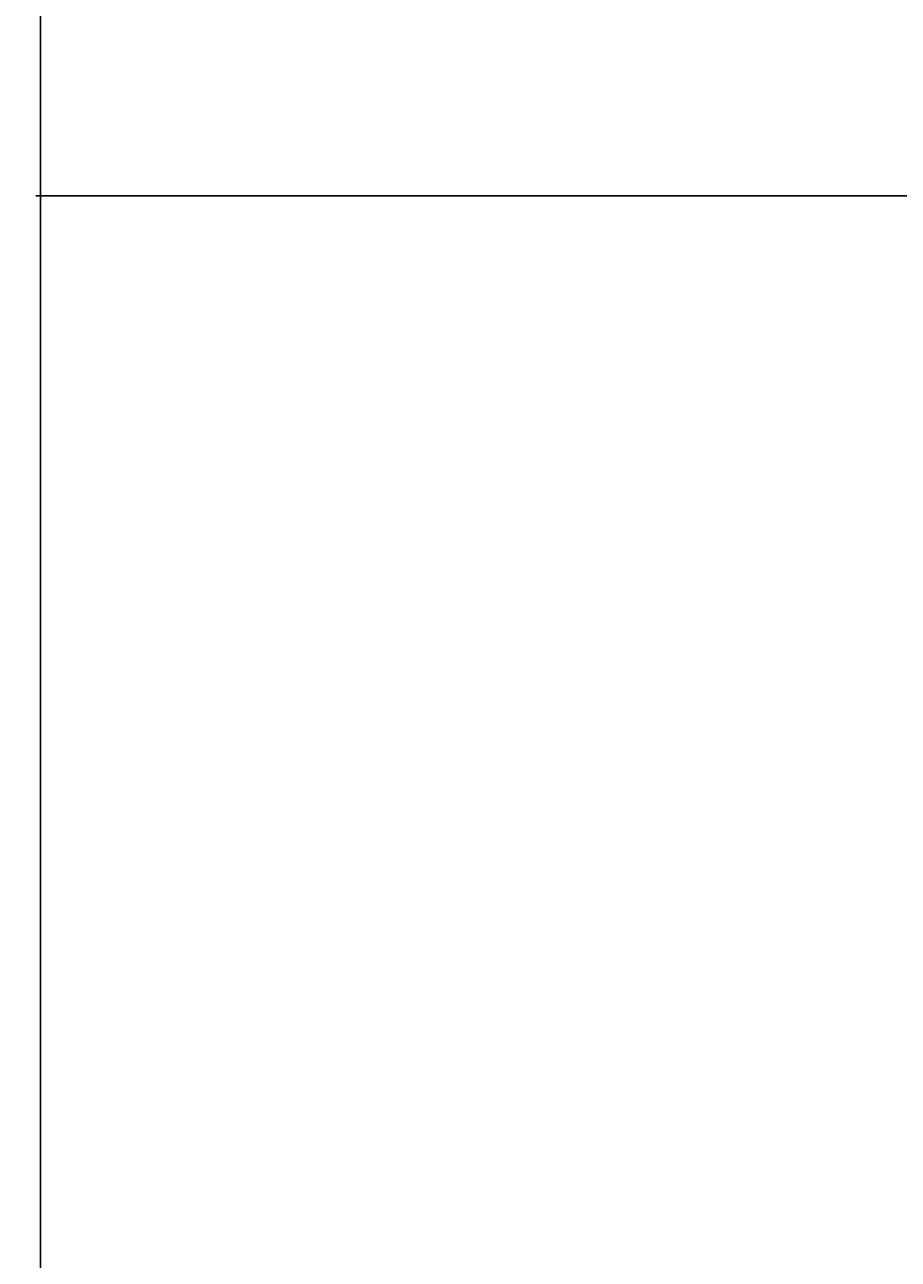
# Model space of a CAD drawing. Units: inches. Extents: x -301 to 715, y -607 to 364.
# Tile 96 of 141: x 161 to 194, y -124 to -77. Entities that reach past the tile are written whole.
import ezdxf

# ---------------------------------------------------------------- set-up
doc = ezdxf.new("R2010")
doc.units = ezdxf.units.IN
doc.header["$MEASUREMENT"] = 0
doc.layers.add('A-ANNO-DIMS', color=2, linetype='Continuous', lineweight=18)
doc.styles.get("Standard").update_dxf_attribs({"font": 'arial.ttf'})
doc.dimstyles.get("Standard").update_dxf_attribs({"dimtxt": 0.18, "dimasz": 0.18, "dimexe": 0.18, "dimexo": 0.0625, "dimgap": 0.09, "dimtad": 0, "dimtih": 1, "dimtoh": 1, "dimdec": 1, "dimzin": 0, "dimdsep": 46, "dimlunit": 4, "dimtxsty": 'Standard', "dimcen": 0.09, "dimclrd": 3, "dimclre": 4, "dimclrt": 6, "dimadec": 0, "dimazin": 0, "dimtfac": 1, "dimtdec": 1, "dimtofl": 0, "dimtmove": 0, "dimatfit": 3, "dimfxl": 1, "dimtfill": 2, "dimtfillclr": 51, "dimtolj": 1, "dimtzin": 0, "dimarcsym": 0})

# ---------------------------------------------------------------- blocks, each defined once
blk = doc.blocks.new('*D162')
at = {"layer": 'A-ANNO-DIMS', "color": 4, "lineweight": -2, "transparency": 16777216}
for p, q in [((222.328, 320.182), (161.439, 320.182)), ((222.328, -233.818), (161.439, -233.818))]:
    blk.add_line(p, q, dxfattribs=at)
at = {"layer": 'A-ANNO-DIMS', "color": 3, "lineweight": -2, "transparency": 16777216}
for p, q in [((161.619, 320.002), (161.619, 43.364)), ((161.619, -233.638), (161.619, 43))]:
    blk.add_line(p, q, dxfattribs=at)
at = {"layer": 'A-ANNO-DIMS', "color": 3, "transparency": 16777216}
for points in [[(161.589, 320.002), (161.649, 320.002), (161.619, 320.182)], [(161.589, -233.638), (161.649, -233.638), (161.619, -233.818)]]:
    blk.add_solid(points, dxfattribs=at)
at = {"layer": 'Defpoints', "color": 0, "transparency": 16777216}
for p in [(161.619, 320.182), (222.39, 320.182), (222.39, -233.818)]:
    blk.add_point(p, dxfattribs=at)
at = {"layer": 'A-ANNO-DIMS', "color": 6, "transparency": 16777216, "insert": (161.619, 43.182), "char_height": 0.18, "attachment_point": 5, "bg_fill": 1, "box_fill_scale": 1.25, "bg_fill_color": 51, "bg_fill_transparency": 0}
blk.add_mtext('\\A1;46\'-2"', dxfattribs=at)
blk = doc.blocks.new('*D167')
at = {"layer": 'A-ANNO-DIMS', "color": 4, "lineweight": -2, "transparency": 16777216}
for p, q in [((222.328, -83.318), (161.439, -83.318)), ((222.328, -233.818), (161.439, -233.818))]:
    blk.add_line(p, q, dxfattribs=at)
at = {"layer": 'A-ANNO-DIMS', "color": 3, "lineweight": -2, "transparency": 16777216}
for p, q in [((161.619, -83.498), (161.619, -158.385)), ((161.619, -233.638), (161.619, -158.751))]:
    blk.add_line(p, q, dxfattribs=at)
at = {"layer": 'A-ANNO-DIMS', "color": 3, "transparency": 16777216}
for points in [[(161.589, -83.498), (161.649, -83.498), (161.619, -83.318)], [(161.589, -233.638), (161.649, -233.638), (161.619, -233.818)]]:
    blk.add_solid(points, dxfattribs=at)
at = {"layer": 'Defpoints', "color": 0, "transparency": 16777216}
for p in [(161.619, -83.318), (222.39, -83.318), (222.39, -233.818)]:
    blk.add_point(p, dxfattribs=at)
at = {"layer": 'A-ANNO-DIMS', "color": 6, "transparency": 16777216, "insert": (161.619, -158.568), "char_height": 0.18, "attachment_point": 5, "bg_fill": 1, "box_fill_scale": 1.25, "bg_fill_color": 51, "bg_fill_transparency": 0}
blk.add_mtext('\\A1;12\'-6 1/2"', dxfattribs=at)
blk = doc.blocks.new('*D168')
at = {"layer": 'A-ANNO-DIMS', "color": 4, "lineweight": -2, "transparency": 16777216}
for p, q in [((222.328, 55.682), (161.439, 55.682)), ((222.328, -83.318), (161.439, -83.318))]:
    blk.add_line(p, q, dxfattribs=at)
at = {"layer": 'A-ANNO-DIMS', "color": 3, "lineweight": -2, "transparency": 16777216}
for p, q in [((161.619, 55.502), (161.619, -13.637)), ((161.619, -83.138), (161.619, -13.998))]:
    blk.add_line(p, q, dxfattribs=at)
at = {"layer": 'A-ANNO-DIMS', "color": 3, "transparency": 16777216}
for points in [[(161.589, 55.502), (161.649, 55.502), (161.619, 55.682)], [(161.589, -83.138), (161.649, -83.138), (161.619, -83.318)]]:
    blk.add_solid(points, dxfattribs=at)
at = {"layer": 'Defpoints', "color": 0, "transparency": 16777216}
for p in [(161.619, 55.682), (222.39, 55.682), (222.39, -83.318)]:
    blk.add_point(p, dxfattribs=at)
at = {"layer": 'A-ANNO-DIMS', "color": 6, "transparency": 16777216, "insert": (161.619, -13.818), "char_height": 0.18, "attachment_point": 5, "bg_fill": 1, "box_fill_scale": 1.25, "bg_fill_color": 51, "bg_fill_transparency": 0}
blk.add_mtext('\\A1;11\'-7"', dxfattribs=at)

msp = doc.modelspace()

# ---------------------------------------------------------------- dimensions: what is measured, and where the dimension line sits
at = {"layer": 'A-ANNO-DIMS'}
for base, p1, p2, picture, middle in [((161.619, 320.182), (222.39, -233.818), (222.39, 320.182), '*D162', (161.619, 43.182)), ((161.619, 55.682), (222.39, -83.318), (222.39, 55.682), '*D168', (161.619, -13.818)), ((161.619, -83.318), (222.39, -233.818), (222.39, -83.318), '*D167', (161.619, -158.568))]:
    dim = msp.add_linear_dim(base=base, p1=p1, p2=p2, angle=90, dimstyle='Standard', override={"dimdec": 1, "dimlfac": 1, "dimrnd": 0, "dimzin": 1, "dimdsep": 46, "dimlunit": 4, "dimfrac": 2}, dxfattribs=at)
    dim.commit()
    dim.dimension.update_dxf_attribs({"geometry": picture, "text_midpoint": middle})

doc.saveas('drawing.dxf')
